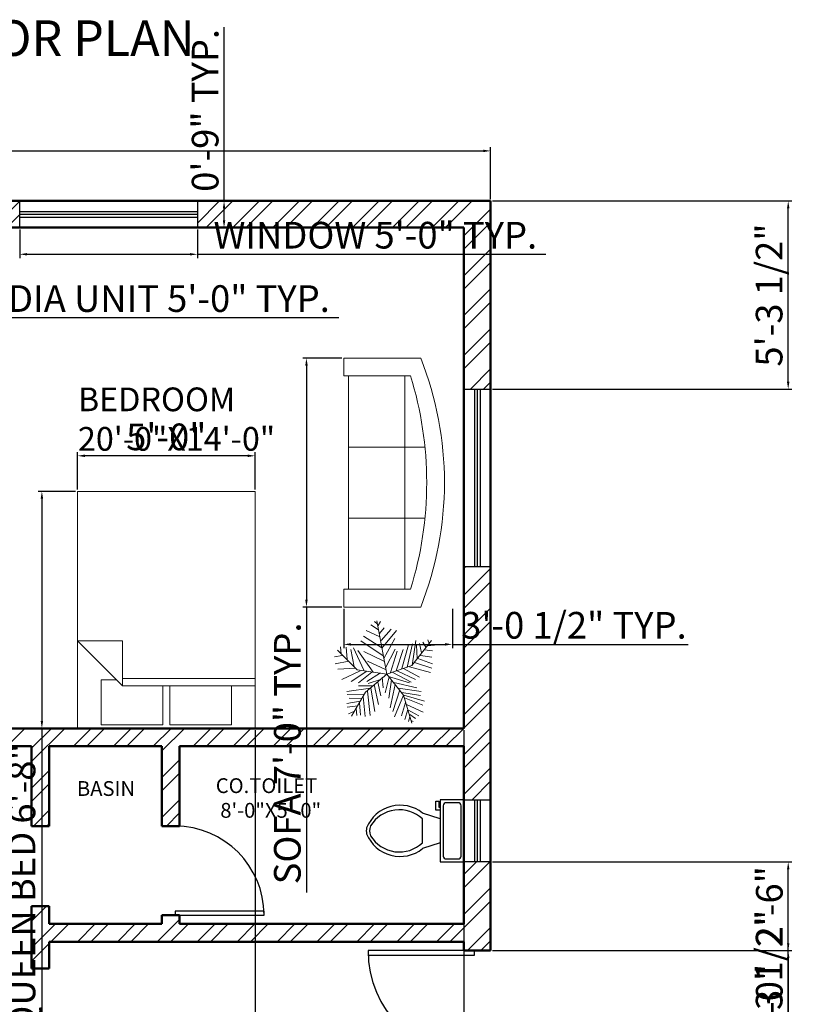
# Model space of a CAD drawing. Units: inches. Extents: x 635 to 1184, y 1837 to 2697.
# Tile 6 of 6: x 916 to 1184, y 2356 to 2688. Entities that reach past the tile are written whole.
import ezdxf

# ---------------------------------------------------------------- set-up
doc = ezdxf.new("R2010")
doc.units = ezdxf.units.IN
for name, color, linetype, lineweight in [('A-ANNO-DIMS', 2, 'Continuous', 18), ('A-ANNO-TEXT', 7, 'Continuous', 25), ('A-AREA-IDEN', 7, 'Continuous', 25), ('A-DOOR', 4, 'Continuous', 25), ('A-FLOR-FIXT', 8, 'Continuous', 25), ('A-FURN', 8, 'Continuous', 18), ('A-GLAZ', 244, 'Continuous', 25), ('A-WALL', 7, 'Continuous', 50), ('A-WALL-PATT', 252, 'Continuous', 13), ('L-PLNT', 94, 'Continuous', 13)]:
    doc.layers.add(name, color=color, linetype=linetype, lineweight=lineweight)
doc.styles.get("Standard").update_dxf_attribs({"font": 'arial.ttf'})
doc.dimstyles.new('ISO-25', dxfattribs={"dimtxt": 9, "dimasz": 2.5, "dimexe": 1.25, "dimexo": 0.625, "dimtad": 1, "dimlunit": 3, "dimtxsty": 'Standard', "dimcen": 2.5, "dimadec": 0, "dimazin": 0, "dimtfac": 1, "dimtmove": 0, "dimatfit": 3, "dimfxl": 1, "dimarcsym": 0})

# ---------------------------------------------------------------- blocks, each defined once
blk = doc.blocks.new('*U4')
for p, q in [((0, 0), (0, -6)), ((-40, 0), (-40, -6))]:
    blk.add_line(p, q)
blk.add_lwpolyline([(0, 0), (0, 40), (-1.75, 40), (-1.75, 0)], close=True)
blk.add_arc((0, 0), 40, 90, 180)
blk = doc.blocks.new('*U6')
for p, q in [((0, 0), (0, 6)), ((40, 0), (40, 6))]:
    blk.add_line(p, q)
blk.add_lwpolyline([(0, 0), (0, -40), (1.75, -40), (1.75, 0)], close=True)
blk.add_arc((0, 0), 40, 270, 0)
blk = doc.blocks.new('*U8')
for p, q in [((9.5, -6), (9.5, -2)), ((-10, -8.5), (-8, -8.5)), ((-10, -9.5), (-10, -8.5)), ((-7, -9.5), (-10, -9.5)), ((-8, -8.5), (-8, -8)), ((-7, -8), (-7, -9.5)), ((-4, -8), (-6, -14)), ((4, -8), (6, -14)), ((4, -14), (-4, -14))]:
    blk.add_line(p, q)
blk.add_lwpolyline([(10.5, -8), (10.5, 0), (-10.5, 0), (-10.5, -8)], close=True)
for points in [[(-9.5, -2), (-9.5, -6)], [(8.5, -1), (-8.5, -1)], [(-8.5, -7), (8.5, -7)]]:
    blk.add_lwpolyline(points)
for centre, radius, start, end in [((-8.62, -1.88), 0.884, 81.8699, 188.1301), ((8.62, -1.88), 0.884, 351.8699, 98.1301), ((-8.62, -6.12), 0.884, 171.8699, 278.1301), ((8.62, -6.12), 0.884, 261.8699, 8.1301), ((3.52, -21.58), 12.17, 141.4691, 247.9714), ((4.2, -21.82), 11.33, 136.3677, 238.9468), ((-3.52, -21.58), 12.17, 292.0284, 38.5307), ((-4.2, -21.82), 11.33, 301.053, 43.6321), ((0, -27.88), 4, 245.7318, 294.2682), ((0, -29), 4, 254.8605, 285.1395)]:
    blk.add_arc(centre, radius, start, end)
blk = doc.blocks.new('Bed - Queen')
for p, q in [((0, -80.00003), (0, 0)), ((0, 0), (59.99999, 0)), ((59.99999, 0), (59.99999, -80.00003)), ((7.99999, -1.2), (28.79998, -1.2)), ((7.99999, -14.4), (7.99999, -1.2)), ((28.79998, -1.2), (28.79998, -14.4)), ((31.19999, -1.2), (51.99999, -1.2)), ((31.19999, -14.4), (31.19999, -1.2)), ((51.99999, -1.2), (51.99999, -16.4)), ((0, -14.4), (44.8, -14.4)), ((59.99999, -29.6), (44.8, -14.4)), ((44.8, -14.4), (44.8, -29.6)), ((51.99999, -16.4), (46.79936, -16.4)), ((44.8, -16.8), (0, -16.8)), ((44.8, -29.6), (59.99999, -29.6)), ((59.99999, -80.00003), (0, -80.00003))]:
    blk.add_line(p, q)
blk = doc.blocks.new('Sofa - Roundback 7 ft.')
for p, q in [((-12.00002, -32.4421), (-12.00003, -6.5971)), ((11.99997, -32.4421), (11.99998, -6.5971)), ((-36.000027, -34), (-36.000027, -11.4696)), ((35.99998, -34), (35.99998, -11.4696)), ((-35.999844, -13.3819), (35.9998, -13.3819)), ((-36.000027, -32.4421), (35.99998, -32.4421))]:
    blk.add_line(p, q)
for points in [[(-36.000027, -34), (-42.000027, -34), (-42.000027, -8)], [(41.99998, -8), (41.99998, -34), (35.99998, -34)]]:
    blk.add_lwpolyline(points)
for centre, radius, start, end in [((0, -114.25), 114.25, 68.43141, 111.5686), ((-0.00001, -127.1968), 121.1968, 72.72033, 107.2797)]:
    blk.add_arc(centre, radius, start, end)
blk = doc.blocks.new('*U15')
for p, q in [((-8.737, 47.138), (-17.069, 52.711)), ((-10.186, 53.64), (-13.084, 55.962)), ((0, 0), (-10.5, 57)), ((-9.099, 51.782), (-6.563, 55.962)), ((-7.288, 39.707), (-21.778, 46.673)), ((-7.65, 43.423), (-2.578, 49.46)), ((-5.839, 35.992), (4.667, 48.067)), ((-5.114, 27.632), (10.463, 46.673)), ((-3.665, 19.273), (-27.574, 35.527)), ((-5.114, 28.097), (-24.676, 40.636)), ((-2.941, 16.486), (8.652, 37.85)), ((22.055, 7.198), (27.489, 32.277)), ((27, 9), (48, 36)), ((27.127, 9.056), (31.112, 35.992)), ((35.096, 32.741), (37.27, 22.524)), ((38.719, 34.134), (41.979, 28.561)), ((44.153, 36.456), (45.239, 32.741)), ((-31.5, 4.5), (-52.5, 25.5)), ((-48.585, 21.131), (-49.309, 29.026)), ((-43.513, 28.561), (-42.427, 15.558)), ((-38.442, 26.239), (-34.819, 7.663)), ((-35.544, 28.097), (-24.314, 3.947)), ((-14.533, 2.09), (-30.834, 25.31)), ((-24.314, 23.917), (-2.941, 13.7)), ((-1.129, 6.734), (9.014, 26.704)), ((3.942, 1.625), (11.187, 24.381)), ((10.101, 3.483), (17.708, 26.239)), ((16.259, 5.805), (23.142, 31.348)), ((31.836, 30.883), (32.561, 16.486)), ((40.53, 25.775), (48.862, 24.846)), ((43.791, 29.954), (51.036, 30.883)), ((-47.498, 19.737), (-55.83, 18.344)), ((-40.615, 13.7), (-55.105, 10.913)), ((-20.691, 13.7), (-1.129, 4.876)), ((29.662, 12.307), (48.137, 6.269)), ((33.285, 16.486), (48.862, 10.913)), ((36.183, 19.737), (48.137, 17.88)), ((-33.37, 6.269), (-52.207, 5.34)), ((-28.299, 3.483), (-47.86, -5.805)), ((-21.416, 3.018), (-38.079, -8.128)), ((0, 0), (-31.5, 4.5)), ((-15.982, 2.09), (-30.11, -9.521)), ((0, 0), (-22.5, -19.5)), ((-6.563, 1.161), (-21.416, -8.128)), ((0, 0), (27, 9)), ((0, 0), (18, -22.5)), ((6.478, 1.625), (26.04, -8.592)), ((11.187, 3.483), (30.749, -5.805)), ((18.07, 5.805), (35.096, -3.483)), ((24.229, 7.663), (46.688, 1.625)), ((-6.563, -5.805), (-19.967, -9.985)), ((-9.461, -8.592), (-6.201, -23.453)), ((-4.752, -3.483), (-3.665, -14.629)), ((2.493, -3.019), (-1.491, -20.202)), ((1.769, -2.555), (24.229, -9.521)), ((5.029, -6.27), (2.131, -25.775)), ((7.565, -9.056), (32.198, -14.629)), ((-17.431, -15.094), (-42.789, -18.809)), ((-22.5, -19.5), (-37.5, -45)), ((-15.257, -12.772), (-30.11, -12.772)), ((-20.691, -18.345), (-17.793, -44.352)), ((-17.069, -15.094), (-12.721, -40.172)), ((-13.446, -11.378), (-8.737, -32.741)), ((9.014, -11.378), (3.58, -35.992)), ((14.085, -16.951), (6.478, -40.172)), ((12.274, -15.094), (36.907, -18.809)), ((16.259, -19.738), (36.183, -22.989)), ((-28.299, -29.026), (-42.789, -31.348)), ((-24.314, -21.596), (-42.427, -22.06)), ((-26.849, -26.24), (-40.253, -25.775)), ((-29.023, -30.884), (-27.936, -43.887)), ((-25.038, -23.918), (-22.865, -45.281)), ((18.07, -22.524), (8.289, -45.745)), ((20.244, -30.419), (15.897, -44.816)), ((18, -22.5), (27, -52.5)), ((18.433, -22.524), (40.53, -29.026)), ((19.157, -25.311), (38.719, -33.206)), ((-30.834, -34.135), (-42.427, -35.528)), ((-34.457, -39.708), (-40.978, -42.494)), ((-32.646, -36.921), (-31.921, -44.352)), ((22.78, -37.85), (19.519, -48.532)), ((21.331, -32.741), (39.081, -40.636)), ((22.78, -38.314), (34.372, -44.816)), ((24.591, -45.745), (23.142, -50.854)), ((24.591, -43.423), (30.749, -47.603)), ((26.764, -49.925), (28.213, -50.854))]:
    blk.add_line(p, q)
blk = doc.blocks.new('*D18')
at = {"layer": 'A-ANNO-DIMS', "color": 0, "lineweight": -2, "transparency": 16777216}
for p, q in [((714.28, 2627.77), (714.28, 2645.3)), ((1075.28, 2627.77), (1075.28, 2645.3)), ((716.78, 2644.05), (1072.78, 2644.05))]:
    blk.add_line(p, q, dxfattribs=at)
at = {"layer": 'A-ANNO-DIMS', "color": 0, "transparency": 16777216}
for points in [[(716.78, 2644.46), (716.78, 2643.63), (714.28, 2644.05)], [(1072.78, 2644.46), (1072.78, 2643.63), (1075.28, 2644.05)]]:
    blk.add_solid(points, dxfattribs=at)
at = {"layer": 'DEFPOINTS', "color": 0, "transparency": 16777216}
for p in [(1075.28, 2644.05), (714.28, 2627.14), (1075.28, 2627.14)]:
    blk.add_point(p, dxfattribs=at)
at = {"layer": 'A-ANNO-DIMS', "color": 0, "transparency": 16777216, "insert": (894.78, 2649.27), "char_height": 9, "attachment_point": 5}
blk.add_mtext('30\'-1"', dxfattribs=at)
blk = doc.blocks.new('WIN-21IN')
for p, q in [((3.5, 21), (3.5, 0)), ((4.5, 21), (4.5, 0)), ((5.5, 21), (5.5, 0))]:
    blk.add_line(p, q)
blk.add_lwpolyline([(0, 21), (9, 21), (9, 0), (0, 0)], close=True)
blk = doc.blocks.new('WIN-60IN')
for p, q in [((0, 5.5), (60, 5.5)), ((0, 4.5), (60, 4.5)), ((0, 3.5), (60, 3.5))]:
    blk.add_line(p, q)
blk.add_lwpolyline([(0, 9), (60, 9), (60, 0), (0, 0)], close=True)
blk = doc.blocks.new('*D23')
at = {"layer": 'A-ANNO-DIMS', "color": 0, "lineweight": -2, "transparency": 16777216}
for p, q in [((916.28, 2617.52), (916.28, 2607.89)), ((976.28, 2617.52), (976.28, 2607.89)), ((918.78, 2609.14), (973.78, 2609.14)), ((976.28, 2609.14), (1093.92, 2609.14))]:
    blk.add_line(p, q, dxfattribs=at)
at = {"layer": 'A-ANNO-DIMS', "color": 0, "transparency": 16777216}
for points in [[(918.78, 2609.56), (918.78, 2608.73), (916.28, 2609.14)], [(973.78, 2609.56), (973.78, 2608.73), (976.28, 2609.14)]]:
    blk.add_solid(points, dxfattribs=at)
at = {"layer": 'DEFPOINTS', "color": 0, "transparency": 16777216}
for p in [(916.28, 2618.14), (976.28, 2618.14), (976.28, 2609.14)]:
    blk.add_point(p, dxfattribs=at)
at = {"layer": 'A-ANNO-DIMS', "color": 0, "transparency": 16777216, "insert": (1036.35, 2614.42), "char_height": 9, "attachment_point": 5}
blk.add_mtext('WINDOW 5\'-0" TYP.', dxfattribs=at)
blk = doc.blocks.new('*D24')
at = {"layer": 'A-ANNO-DIMS', "color": 0, "lineweight": -2, "transparency": 16777216}
for p, q in [((985.28, 2627.14), (985.28, 2685.75)), ((976.91, 2627.14), (986.53, 2627.14)), ((985.28, 2620.64), (985.28, 2624.64)), ((976.91, 2618.14), (986.53, 2618.14))]:
    blk.add_line(p, q, dxfattribs=at)
at = {"layer": 'A-ANNO-DIMS', "color": 0, "transparency": 16777216}
for points in [[(984.87, 2624.64), (985.7, 2624.64), (985.28, 2627.14)], [(984.87, 2620.64), (985.7, 2620.64), (985.28, 2618.14)]]:
    blk.add_solid(points, dxfattribs=at)
at = {"layer": 'DEFPOINTS', "color": 0, "transparency": 16777216}
for p in [(976.28, 2627.14), (985.28, 2627.14), (976.28, 2618.14)]:
    blk.add_point(p, dxfattribs=at)
at = {"layer": 'A-ANNO-DIMS', "color": 0, "transparency": 16777216, "insert": (980.06, 2657.7), "char_height": 9, "attachment_point": 5, "rotation": 90}
blk.add_mtext('0\'-9" TYP.', dxfattribs=at)
blk = doc.blocks.new('*D27')
at = {"layer": 'A-ANNO-DIMS', "color": 0, "lineweight": -2, "transparency": 16777216}
for p, q in [((1025.07, 2574.1), (1011.84, 2574.1)), ((1013.09, 2571.6), (1013.09, 2492.6)), ((1025.07, 2490.1), (1011.84, 2490.1)), ((1013.09, 2490.1), (1013.09, 2393.81))]:
    blk.add_line(p, q, dxfattribs=at)
at = {"layer": 'A-ANNO-DIMS', "color": 0, "transparency": 16777216}
for points in [[(1012.68, 2571.6), (1013.51, 2571.6), (1013.09, 2574.1)], [(1012.68, 2492.6), (1013.51, 2492.6), (1013.09, 2490.1)]]:
    blk.add_solid(points, dxfattribs=at)
at = {"layer": 'DEFPOINTS', "color": 0, "transparency": 16777216}
for p in [(1025.69, 2574.1), (1013.09, 2490.1), (1025.69, 2490.1)]:
    blk.add_point(p, dxfattribs=at)
at = {"layer": 'A-ANNO-DIMS', "color": 0, "transparency": 16777216, "insert": (1007.81, 2440.71), "char_height": 9, "attachment_point": 5, "rotation": 90}
blk.add_mtext('SOFA 7\'-0" TYP.', dxfattribs=at)
blk = doc.blocks.new('*D28')
at = {"layer": 'A-ANNO-DIMS', "color": 0, "lineweight": -2, "transparency": 16777216}
for p, q in [((1025.69, 2489.48), (1025.69, 2476.25)), ((1062.36, 2489.48), (1062.36, 2476.25)), ((1028.19, 2477.5), (1059.86, 2477.5)), ((1062.36, 2477.5), (1141.93, 2477.5))]:
    blk.add_line(p, q, dxfattribs=at)
at = {"layer": 'A-ANNO-DIMS', "color": 0, "transparency": 16777216}
for points in [[(1028.19, 2477.92), (1028.19, 2477.08), (1025.69, 2477.5)], [(1059.86, 2477.92), (1059.86, 2477.08), (1062.36, 2477.5)]]:
    blk.add_solid(points, dxfattribs=at)
at = {"layer": 'DEFPOINTS', "color": 0, "transparency": 16777216}
for p in [(1025.69, 2490.1), (1062.36, 2490.1), (1062.36, 2477.5)]:
    blk.add_point(p, dxfattribs=at)
at = {"layer": 'A-ANNO-DIMS', "color": 0, "transparency": 16777216, "insert": (1103.4, 2482.78), "char_height": 9, "attachment_point": 5}
blk.add_mtext('3\'-0 1/2" TYP.', dxfattribs=at)
blk = doc.blocks.new('*D29')
at = {"layer": 'A-ANNO-DIMS', "color": 0, "lineweight": -2, "transparency": 16777216}
for p, q in [((829.66, 2596.18), (829.66, 2586.56)), ((889.66, 2596.18), (889.66, 2586.56)), ((832.16, 2587.81), (887.16, 2587.81)), ((889.66, 2587.81), (1024, 2587.81))]:
    blk.add_line(p, q, dxfattribs=at)
at = {"layer": 'A-ANNO-DIMS', "color": 0, "transparency": 16777216}
for points in [[(832.16, 2588.23), (832.16, 2587.39), (829.66, 2587.81)], [(887.16, 2588.23), (887.16, 2587.39), (889.66, 2587.81)]]:
    blk.add_solid(points, dxfattribs=at)
at = {"layer": 'DEFPOINTS', "color": 0, "transparency": 16777216}
for p in [(829.66, 2596.81), (889.66, 2596.81), (889.66, 2587.81)]:
    blk.add_point(p, dxfattribs=at)
at = {"layer": 'A-ANNO-DIMS', "color": 0, "transparency": 16777216, "insert": (958.08, 2593.03), "char_height": 9, "attachment_point": 5}
blk.add_mtext('MEDIA UNIT 5\'-0" TYP.', dxfattribs=at)
blk = doc.blocks.new('*D35')
at = {"layer": 'A-ANNO-DIMS', "color": 0, "lineweight": -2, "transparency": 16777216}
for p, q in [((935.16, 2529.14), (922.53, 2529.14)), ((923.78, 2526.64), (923.78, 2451.64)), ((935.16, 2449.14), (922.53, 2449.14)), ((923.78, 2449.14), (923.78, 2343.94))]:
    blk.add_line(p, q, dxfattribs=at)
at = {"layer": 'A-ANNO-DIMS', "color": 0, "transparency": 16777216}
for points in [[(923.37, 2526.64), (924.2, 2526.64), (923.78, 2529.14)], [(923.37, 2451.64), (924.2, 2451.64), (923.78, 2449.14)]]:
    blk.add_solid(points, dxfattribs=at)
at = {"layer": 'DEFPOINTS', "color": 0, "transparency": 16777216}
for p in [(935.78, 2529.14), (923.78, 2449.14), (935.78, 2449.14)]:
    blk.add_point(p, dxfattribs=at)
at = {"layer": 'A-ANNO-DIMS', "color": 0, "transparency": 16777216, "insert": (918.23, 2395.29), "char_height": 9, "attachment_point": 5, "rotation": 90}
blk.add_mtext('QUEEN BED 6\'-8"', dxfattribs=at)
blk = doc.blocks.new('*D36')
at = {"layer": 'A-ANNO-DIMS', "color": 0, "lineweight": -2, "transparency": 16777216}
for p, q in [((935.78, 2529.77), (935.78, 2542.39)), ((995.78, 2529.77), (995.78, 2542.39)), ((993.28, 2541.14), (938.28, 2541.14))]:
    blk.add_line(p, q, dxfattribs=at)
at = {"layer": 'A-ANNO-DIMS', "color": 0, "transparency": 16777216}
for points in [[(938.28, 2541.56), (938.28, 2540.73), (935.78, 2541.14)], [(993.28, 2541.56), (993.28, 2540.73), (995.78, 2541.14)]]:
    blk.add_solid(points, dxfattribs=at)
at = {"layer": 'DEFPOINTS', "color": 0, "transparency": 16777216}
for p in [(935.78, 2541.14), (935.78, 2529.14), (995.78, 2529.14)]:
    blk.add_point(p, dxfattribs=at)
at = {"layer": 'A-ANNO-DIMS', "color": 0, "transparency": 16777216, "insert": (965.78, 2546.36), "char_height": 9, "attachment_point": 5}
blk.add_mtext('5\'-0"', dxfattribs=at)
blk = doc.blocks.new('*D45')
at = {"layer": 'A-ANNO-DIMS', "color": 0, "lineweight": -2, "transparency": 16777216}
for p, q in [((1075.91, 2627.14), (1176.99, 2627.14)), ((1175.74, 2566.14), (1175.74, 2624.64)), ((1075.91, 2563.64), (1176.99, 2563.64))]:
    blk.add_line(p, q, dxfattribs=at)
at = {"layer": 'A-ANNO-DIMS', "color": 0, "transparency": 16777216}
for points in [[(1175.32, 2624.64), (1176.15, 2624.64), (1175.74, 2627.14)], [(1175.32, 2566.14), (1176.15, 2566.14), (1175.74, 2563.64)]]:
    blk.add_solid(points, dxfattribs=at)
at = {"layer": 'DEFPOINTS', "color": 0, "transparency": 16777216}
for p in [(1075.28, 2627.14), (1175.74, 2627.14), (1075.28, 2563.64)]:
    blk.add_point(p, dxfattribs=at)
at = {"layer": 'A-ANNO-DIMS', "color": 0, "transparency": 16777216, "insert": (1170.46, 2595.39), "char_height": 9, "attachment_point": 5, "rotation": 90}
blk.add_mtext('5\'-3 1/2"', dxfattribs=at)
blk = doc.blocks.new('*D51')
at = {"layer": 'A-ANNO-DIMS', "color": 0, "lineweight": -2, "transparency": 16777216}
for p, q in [((1075.91, 2374.14), (1176.99, 2374.14)), ((1175.74, 2371.64), (1175.74, 2340.64)), ((1075.91, 2338.14), (1176.99, 2338.14))]:
    blk.add_line(p, q, dxfattribs=at)
at = {"layer": 'A-ANNO-DIMS', "color": 0, "transparency": 16777216}
for points in [[(1175.32, 2371.64), (1176.15, 2371.64), (1175.74, 2374.14)], [(1175.32, 2340.64), (1176.15, 2340.64), (1175.74, 2338.14)]]:
    blk.add_solid(points, dxfattribs=at)
at = {"layer": 'DEFPOINTS', "color": 0, "transparency": 16777216}
for p in [(1075.28, 2374.14), (1075.28, 2338.14), (1175.74, 2338.14)]:
    blk.add_point(p, dxfattribs=at)
at = {"layer": 'A-ANNO-DIMS', "color": 0, "transparency": 16777216, "insert": (1170.51, 2356.14), "char_height": 9, "attachment_point": 5, "rotation": 90}
blk.add_mtext('3\'-0"', dxfattribs=at)
blk = doc.blocks.new('*D54')
at = {"layer": 'A-ANNO-DIMS', "color": 0, "lineweight": -2, "transparency": 16777216}
for p, q in [((1175.74, 2338.14), (1175.74, 2386.94)), ((1075.91, 2338.14), (1176.99, 2338.14)), ((1175.74, 2312.94), (1175.74, 2335.64)), ((1075.91, 2310.44), (1176.99, 2310.44))]:
    blk.add_line(p, q, dxfattribs=at)
at = {"layer": 'A-ANNO-DIMS', "color": 0, "transparency": 16777216}
for points in [[(1175.32, 2335.64), (1176.15, 2335.64), (1175.74, 2338.14)], [(1175.32, 2312.94), (1176.15, 2312.94), (1175.74, 2310.44)]]:
    blk.add_solid(points, dxfattribs=at)
at = {"layer": 'DEFPOINTS', "color": 0, "transparency": 16777216}
for p in [(1075.28, 2338.14), (1175.74, 2338.14), (1075.28, 2310.44)]:
    blk.add_point(p, dxfattribs=at)
at = {"layer": 'A-ANNO-DIMS', "color": 0, "transparency": 16777216, "insert": (1170.46, 2363.79), "char_height": 9, "attachment_point": 5, "rotation": 90}
blk.add_mtext('2\'-3 1/2"', dxfattribs=at)
blk = doc.blocks.new('*D55')
at = {"layer": 'A-ANNO-DIMS', "color": 0, "lineweight": -2, "transparency": 16777216}
for p, q in [((1075.91, 2404.07), (1176.99, 2404.07)), ((1175.74, 2376.64), (1175.74, 2401.57)), ((1075.91, 2374.14), (1176.99, 2374.14))]:
    blk.add_line(p, q, dxfattribs=at)
at = {"layer": 'A-ANNO-DIMS', "color": 0, "transparency": 16777216}
for points in [[(1175.32, 2401.57), (1176.15, 2401.57), (1175.74, 2404.07)], [(1175.32, 2376.64), (1176.15, 2376.64), (1175.74, 2374.14)]]:
    blk.add_solid(points, dxfattribs=at)
at = {"layer": 'DEFPOINTS', "color": 0, "transparency": 16777216}
for p in [(1075.28, 2404.07), (1175.74, 2404.07), (1075.28, 2374.14)]:
    blk.add_point(p, dxfattribs=at)
at = {"layer": 'A-ANNO-DIMS', "color": 0, "transparency": 16777216, "insert": (1170.52, 2389.11), "char_height": 9, "attachment_point": 5, "rotation": 90}
blk.add_mtext('2\'-6"', dxfattribs=at)
blk = doc.blocks.new('*D63')
at = {"layer": 'A-ANNO-DIMS', "color": 0, "lineweight": -2, "transparency": 16777216}
for p, q in [((995.78, 2448.52), (995.78, 1843.99)), ((1066.28, 2448.52), (1066.28, 1843.99)), ((998.28, 1845.24), (1063.78, 1845.24))]:
    blk.add_line(p, q, dxfattribs=at)
at = {"layer": 'A-ANNO-DIMS', "color": 0, "transparency": 16777216}
for points in [[(998.28, 1845.65), (998.28, 1844.82), (995.78, 1845.24)], [(1063.78, 1845.65), (1063.78, 1844.82), (1066.28, 1845.24)]]:
    blk.add_solid(points, dxfattribs=at)
at = {"layer": 'DEFPOINTS', "color": 0, "transparency": 16777216}
for p in [(995.78, 2449.14), (1066.28, 2449.14), (1066.28, 1845.24)]:
    blk.add_point(p, dxfattribs=at)
at = {"layer": 'A-ANNO-DIMS', "color": 0, "transparency": 16777216, "insert": (1031.03, 1850.52), "char_height": 9, "attachment_point": 5}
blk.add_mtext('5\'-10 1/2"', dxfattribs=at)

msp = doc.modelspace()

# ---------------------------------------------------------------- hatches: boundary and pattern name
at = {"layer": 'A-WALL-PATT'}
h = msp.add_hatch(dxfattribs=at)
h.set_pattern_fill('ANSI32', color=256)
h.paths.add_polyline_path([(723.282, 2313.142), (714.282, 2313.142), (714.282, 2234.142), (718.782, 2234.142), (723.282, 2234.142), (723.282, 2237.142), (779.782, 2237.142), (779.782, 2243.142), (723.282, 2243.142)])
h.paths.add_polyline_path([(926.282, 2320.142), (920.282, 2320.142), (920.282, 2243.142), (845.782, 2243.142), (845.782, 2237.142), (920.282, 2237.142), (920.282, 2093.142), (860.282, 2093.142), (860.282, 2165.142), (854.282, 2165.142), (854.282, 2093.142), (818.782, 2093.142), (818.782, 2084.142), (929.282, 2084.142), (929.282, 2156.142), (932.282, 2156.142), (932.282, 2165.142), (926.282, 2165.142)])
h.paths.add_polyline_path([(1075.282, 2250.443), (1066.282, 2250.443), (1066.282, 2233.442), (1075.282, 2233.442)])
h.paths.add_polyline_path([(1075.282, 2173.442), (1066.282, 2173.442), (1066.282, 2165.142), (1057.782, 2165.142), (1057.782, 2156.142), (1075.282, 2156.142)])
h.paths.add_polyline_path([(997.782, 2165.142), (980.282, 2165.142), (980.282, 2156.142), (997.782, 2156.142)])
h.paths.add_polyline_path([(1075.282, 2338.142), (1066.282, 2338.142), (1066.282, 2310.443), (1075.282, 2310.443)])
h.paths.add_polyline_path([(758.782, 2093.142), (723.282, 2093.142), (723.282, 2154.642), (714.282, 2154.642), (714.282, 2084.142), (758.782, 2084.142)])
h.paths.add_polyline_path([(723.282, 2204.142), (714.282, 2204.142), (714.282, 2175.642), (723.282, 2175.642)])
h.paths.add_polyline_path([(1075.282, 2404.069), (1066.282, 2404.069), (1066.282, 2383.142), (970.282, 2383.142), (970.282, 2386.142), (964.282, 2386.142), (964.282, 2383.142), (926.282, 2383.142), (926.282, 2389.142), (920.282, 2389.142), (920.282, 2368.142), (926.282, 2368.142), (926.282, 2377.142), (1066.282, 2377.142), (1066.282, 2374.142), (1075.282, 2374.142)])
h.paths.add_polyline_path([(926.282, 2443.142), (964.282, 2443.142), (964.282, 2416.142), (970.282, 2416.142), (970.282, 2443.142), (1066.282, 2443.142), (1066.282, 2425.069), (1075.282, 2425.069), (1075.282, 2503.642), (1066.282, 2503.642), (1066.282, 2449.142), (865.282, 2449.142), (865.282, 2443.142), (920.282, 2443.142), (920.282, 2416.142), (926.282, 2416.142)])
h.paths.add_polyline_path([(829.282, 2449.142), (826.282, 2449.142), (826.282, 2527.142), (826.282, 2557.642), (820.282, 2557.642), (820.282, 2527.142), (817.282, 2527.142), (817.282, 2521.142), (820.282, 2521.142), (820.282, 2449.142), (723.282, 2449.142), (723.282, 2474.642), (714.282, 2474.642), (714.282, 2373.142), (723.282, 2373.142), (723.282, 2443.142), (829.282, 2443.142)])
h.paths.add_polyline_path([(787.282, 2527.142), (723.282, 2527.142), (723.282, 2618.142), (820.282, 2618.142), (820.282, 2587.642), (826.282, 2587.642), (826.282, 2618.142), (916.282, 2618.142), (916.282, 2627.142), (714.282, 2627.142), (714.282, 2495.642), (723.282, 2495.642), (723.282, 2521.142), (787.282, 2521.142)])
h.paths.add_polyline_path([(1075.282, 2627.142), (976.282, 2627.142), (976.282, 2618.142), (1066.282, 2618.142), (1066.282, 2563.642), (1075.282, 2563.642)])

# ---------------------------------------------------------------- linework, layer by layer
at = {"layer": 'A-WALL'}
for p, q in [((714.282, 2627.142), (1075.282, 2627.142)), ((1075.282, 2627.142), (1075.282, 2374.142)), ((826.282, 2618.142), (1066.282, 2618.142)), ((1066.282, 2618.142), (1066.282, 2449.142)), ((865.282, 2449.142), (1066.282, 2449.142)), ((865.282, 2443.142), (920.282, 2443.142)), ((920.282, 2443.142), (920.282, 2416.142)), ((926.282, 2443.142), (964.282, 2443.142)), ((926.282, 2443.142), (926.282, 2416.142)), ((964.282, 2443.142), (964.282, 2416.142)), ((970.282, 2443.142), (970.282, 2416.142)), ((970.282, 2443.142), (1066.282, 2443.142)), ((1066.282, 2443.142), (1066.282, 2383.142)), ((926.282, 2416.142), (920.282, 2416.142)), ((970.282, 2416.142), (964.282, 2416.142)), ((926.282, 2389.142), (920.282, 2389.142)), ((920.282, 2389.142), (920.282, 2368.142)), ((926.282, 2389.142), (926.282, 2383.142)), ((970.282, 2386.142), (964.282, 2386.142)), ((964.282, 2386.142), (964.282, 2383.142)), ((970.282, 2386.142), (970.282, 2383.142)), ((926.282, 2383.142), (964.282, 2383.142)), ((970.282, 2383.142), (1066.282, 2383.142)), ((926.282, 2377.142), (1066.282, 2377.142)), ((926.282, 2377.142), (926.282, 2368.142)), ((1066.282, 2377.142), (1066.282, 2374.142)), ((1066.282, 2374.142), (1075.282, 2374.142)), ((926.282, 2368.142), (920.282, 2368.142))]:
    msp.add_line(p, q, dxfattribs=at)

# ---------------------------------------------------------------- block references
at = {"layer": 'A-DOOR'}
for name, p, xscale, yscale, zscale, rotation in [('*U6', (968.782, 2386.142), 0.7499999999999997, 0.7499999999999997, 0.7499999999999997, 89.99999999999976), ('*U4', (1069.882, 2374.142), 0.8999999999999996, 0.8999999999999996, 0.8999999999999996, 90)]:
    msp.add_blockref(name, p, dxfattribs=dict(at, xscale=xscale, yscale=yscale, zscale=zscale, rotation=rotation))
at = {"layer": 'A-FLOR-FIXT', "rotation": 270}
msp.add_blockref('*U8', (1066.282, 2414.569), dxfattribs=at)
at = {"layer": 'A-FURN'}
for name, p, rotation in [('Sofa - Roundback 7 ft.', (1059.692, 2532.101), 270), ('Bed - Queen', (995.782, 2449.142), 180)]:
    msp.add_blockref(name, p, dxfattribs=dict(at, rotation=rotation))
at = {"layer": 'A-GLAZ'}
for name, p in [('WIN-60IN', (916.282, 2618.142)), ('WIN-21IN', (1066.282, 2404.069))]:
    msp.add_blockref(name, p, dxfattribs=at)
at = {"layer": 'A-GLAZ', "rotation": 270.0000000000007}
msp.add_blockref('WIN-60IN', (1066.282, 2563.642), dxfattribs=at)
at = {"layer": 'L-PLNT', "xscale": 0.3157050638920436, "yscale": 0.3157050638920436, "zscale": 0.3157050638920436}
msp.add_blockref('*U15', (1040.187, 2467.497), dxfattribs=at)

# ---------------------------------------------------------------- texts
at = {"layer": 'A-ANNO-TEXT', "insert": (805.654, 2688.104), "char_height": 12, "attachment_point": 1}
msp.add_mtext_dynamic_manual_height_columns('GROUND FLOOR PLAN ', width=188.74888, gutter_width=12.5, heights=[0], dxfattribs=at)
at = {"layer": 'A-AREA-IDEN', "attachment_point": 1}
for s, width, insert, char_height in [('BEDROOM\\P20\'-0"X14\'-0"', 65.95878, (935.945, 2564.189), 8), ('CO.TOILET\\P 8\'-0"X5\'-0"', 37.39527, (982.479, 2432.322), 5), ('BASIN', 21.12843, (935.605, 2431.355), 5)]:
    msp.add_mtext_dynamic_manual_height_columns(s, width=width, gutter_width=12.5, heights=[0], dxfattribs=dict(at, insert=insert, char_height=char_height))

# ---------------------------------------------------------------- dimensions: what is measured, and where the dimension line sits
at = {"layer": 'A-ANNO-DIMS'}
for base, p1, p2, angle, text, picture, middle in [((985.282, 2627.142), (976.282, 2618.142), (976.282, 2627.142), 90, '<> TYP.', '*D24', (980.062, 2657.697)), ((1013.092, 2490.101), (1025.692, 2574.101), (1025.692, 2490.101), 270, 'SOFA <> TYP.', '*D27', (1007.81, 2440.705)), ((923.782, 2449.142), (935.782, 2529.142), (935.782, 2449.142), 270, 'QUEEN BED <>', '*D35', (918.227, 2395.289))]:
    dim = msp.add_linear_dim(base=base, p1=p1, p2=p2, angle=angle, text=text, dimstyle='ISO-25', override={"dimdec": 1, "dimlfac": 1, "dimrnd": 0, "dimzin": 1, "dimdsep": 46, "dimlunit": 4, "dimfrac": 2}, dxfattribs=at)
    dim.commit()
    dim.dimension.update_dxf_attribs({"geometry": picture, "text_midpoint": middle})
for base, p1, p2, override, picture, middle in [((1075.282, 2644.045), (714.282, 2627.142), (1075.282, 2627.142), {"dimclrd": 0, "dimclre": 0, "dimclrt": 0}, '*D18', (894.782, 2649.269)), ((1066.282, 1845.237), (995.782, 2449.142), (1066.282, 2449.142), {"dimdec": 1, "dimlfac": 1, "dimrnd": 0, "dimzin": 1, "dimdsep": 46, "dimlunit": 4, "dimfrac": 2}, '*D63', (1031.032, 1850.516))]:
    dim = msp.add_linear_dim(base=base, p1=p1, p2=p2, dimstyle='ISO-25', override=override, dxfattribs=at)
    dim.commit()
    dim.dimension.update_dxf_attribs({"geometry": picture, "text_midpoint": middle})
for base, p1, p2, text, picture, middle in [((976.282, 2609.142), (916.282, 2618.142), (976.282, 2618.142), 'WINDOW <> TYP.', '*D23', (1036.351, 2614.423)), ((889.663, 2587.809), (829.663, 2596.809), (889.663, 2596.809), 'MEDIA UNIT <> TYP.', '*D29', (958.081, 2593.029)), ((1062.358, 2477.501), (1025.692, 2490.101), (1062.358, 2490.101), '<> TYP.', '*D28', (1103.396, 2482.783))]:
    dim = msp.add_linear_dim(base=base, p1=p1, p2=p2, text=text, dimstyle='ISO-25', override={"dimdec": 1, "dimlfac": 1, "dimrnd": 0, "dimzin": 1, "dimdsep": 46, "dimlunit": 4, "dimfrac": 2}, dxfattribs=at)
    dim.commit()
    dim.dimension.update_dxf_attribs({"geometry": picture, "text_midpoint": middle})
for base, p1, p2, angle, picture, middle in [((1175.738, 2627.142), (1075.282, 2563.642), (1075.282, 2627.142), 90, '*D45', (1170.456, 2595.392)), ((935.782, 2541.142), (995.782, 2529.142), (935.782, 2529.142), 180, '*D36', (965.782, 2546.362)), ((1175.738, 2404.069), (1075.282, 2374.142), (1075.282, 2404.069), 90, '*D55', (1170.518, 2389.105)), ((1175.738, 2338.142), (1075.282, 2310.443), (1075.282, 2338.142), 90, '*D54', (1170.456, 2363.791)), ((1175.738, 2338.142), (1075.282, 2374.142), (1075.282, 2338.142), 90, '*D51', (1170.515, 2356.142))]:
    dim = msp.add_linear_dim(base=base, p1=p1, p2=p2, angle=angle, dimstyle='ISO-25', override={"dimdec": 1, "dimlfac": 1, "dimrnd": 0, "dimzin": 1, "dimdsep": 46, "dimlunit": 4, "dimfrac": 2}, dxfattribs=at)
    dim.commit()
    dim.dimension.update_dxf_attribs({"geometry": picture, "text_midpoint": middle})

doc.saveas('drawing.dxf')
